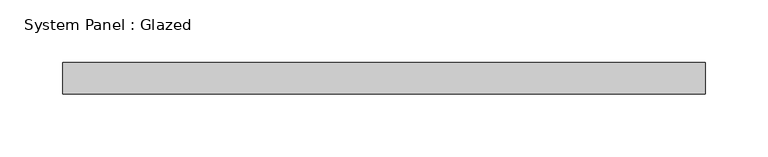
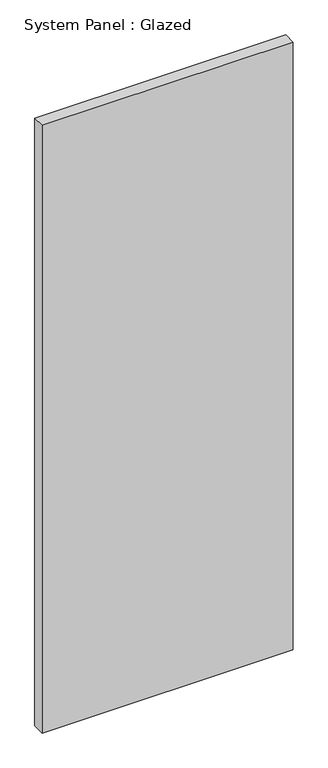
"""IFC4 building model written with IfcOpenShell, lengths in millimetres: plate geometry, System Panel : Glazed."""

from ifc_helpers import new_model, si_unit, origin, origin_with_axes, place, context, project, spatial, polyline, outline, extrude, source, transform, mapped, element, save


def system_panel_glazed_c4277b2e(model_context):
    return source(origin(), model_context, "Body", "SweptSolid", [
        extrude(outline(polyline([(257.175, 19.05), (-257.175, 19.05), (-257.175, 44.45), (257.175, 44.45), (257.175, 19.05)])), origin_with_axes(), (0.0, 0.0, 1.0), 1314.7145247),
    ])


if __name__ == "__main__":
    model = new_model("IFC4")
    model_context = context("Model", 3, world=origin())
    ifc_project = project(units=[si_unit("LENGTHUNIT", "METRE", prefix="MILLI")], contexts=[model_context])
    site = spatial("IfcSite", under=ifc_project)
    building = spatial("IfcBuilding", under=site)
    placement = place(None, origin())
    system_panel_glazed_shape = system_panel_glazed_c4277b2e(model_context)
    element("IfcPlate", 1, ObjectType="System Panel : Glazed", at=placement, inside=building, context=model_context, shape_type="MappedRepresentation", body=[
        mapped(system_panel_glazed_shape, transform((0.0, 0.0, 0.0), x_axis=(1.0, 0.0, 0.0), y_axis=(0.0, 1.0, 0.0), z_axis=(0.0, 0.0, 1.0))),
    ])
    save(model, "model.ifc")

# Revit data of these elements
# Type "System Panel : Glazed"
#   Construction Type Id = "GSP4R"
#   Analytic Construction = "1/8 in Pilkington single glazing"
#   Visual Light Transmittance = 0.9
#   Solar Heat Gain Coefficient = 0.86
#   Heat Transfer Coefficient (U) = 1.18115 BTU/(h·ft²·°F)
#   Define Thermal Properties by = 1
# Element 1 (IfcPlate, "System Panel : Glazed")
#   Materials on its faces: "Glass"
# Materials
#   "Glass": class "Glass", colour RGB 0 128 192, transparency 0.75, Description = "Soda Lime Glass", Cost = 0
